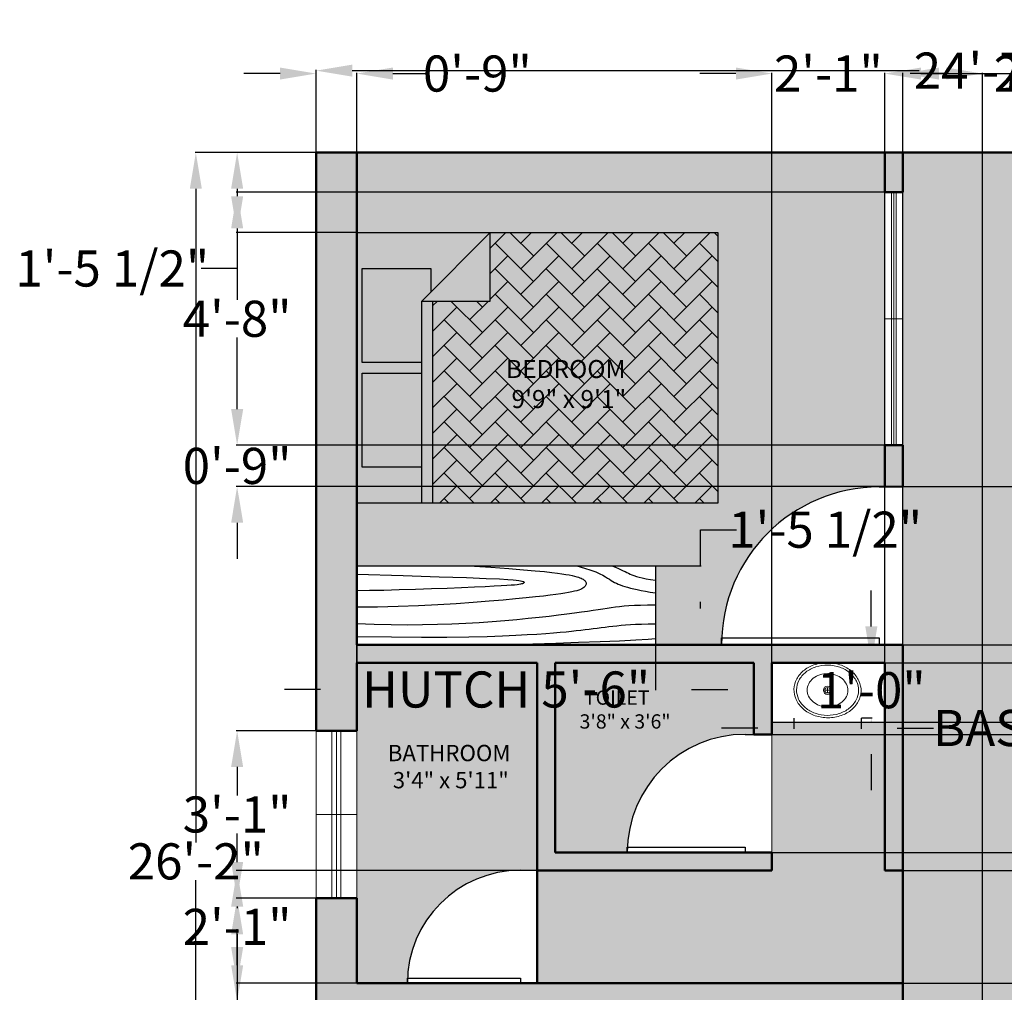
# Model space of a CAD drawing. Units: inches. Extents: x 339 to 824, y 73 to 445.
# Tile 2 of 5: x 387 to 605, y 230 to 445. Entities that reach past the tile are written whole.
import ezdxf

# ---------------------------------------------------------------- set-up
doc = ezdxf.new("R2010")
doc.units = ezdxf.units.IN
doc.header["$MEASUREMENT"] = 0
for name, color, linetype, lineweight in [('A-ANNO-DIMS', 2, 'Continuous', 18), ('A-AREA-IDEN', 7, 'Continuous', 25), ('A-DOOR', 3, 'Continuous', 25), ('A-FLOR-BNDY', 8, 'Continuous', 13), ('A-FLOR-CASE', 7, 'Continuous', 25), ('A-FLOR-FIXT', 9, 'Continuous', 20), ('A-FLOR-PATT', 8, 'Continuous', 13), ('A-FLOR-STRS', 7, 'Continuous', 25), ('A-FLOR-STRS-PATT', 252, 'Continuous', 13), ('A-FURN', 9, 'Continuous', 25), ('A-FURN-FABR-PATT', 7, 'Continuous', 13), ('A-GLAZ', 4, 'Continuous', 18), ('A-WALL', 7, 'Continuous', 50), ('A-WALL-PATT', 1, 'Continuous', 13)]:
    doc.layers.add(name, color=color, linetype=linetype, lineweight=lineweight)
doc.layers.add('A-FURN-PATT', color=251, linetype='Continuous', lineweight=13, true_color=0x6d5f6c)
doc.styles.get("Standard").update_dxf_attribs({"font": 'arial.ttf'})
doc.dimstyles.get("Standard").update_dxf_attribs({"dimtxt": 8, "dimasz": 8, "dimexe": 0.18, "dimexo": 0.0625, "dimgap": 0.09, "dimtad": 0, "dimtih": 1, "dimtoh": 1, "dimdec": 0, "dimzin": 0, "dimdsep": 46, "dimlunit": 3, "dimtxsty": 'Standard', "dimcen": 0.09, "dimadec": 0, "dimazin": 0, "dimtfac": 1, "dimtdec": 0, "dimtofl": 0, "dimtmove": 0, "dimatfit": 3, "dimfxl": 1, "dimtolj": 1, "dimtzin": 0, "dimarcsym": 0})

# ---------------------------------------------------------------- blocks, each defined once
blk = doc.blocks.new('*U2')
for p, q in [((0, 0), (0, -6)), ((40, 0), (40, -6))]:
    blk.add_line(p, q)
blk.add_lwpolyline([(0, 0), (0, 40), (1.75, 40), (1.75, 0)], close=True)
blk.add_arc((0, 0), 40, 0, 90)
blk = doc.blocks.new('Sink - Oval top')
for p, q in [((-1, 0), (1, 0)), ((0, 1), (0, -1))]:
    blk.add_line(p, q)
for points in [[(-12.23, 0.39, 0.117634), (-11.46, -3.36, 0.104469), (-8.88, -6.8, 0.090016), (-5.08, -9.07, 0.08192), (-0.32, -10.02, 0.08192), (4.49, -9.38, 0.090016), (8.42, -7.36, 0.104469), (11.22, -4.09, 0.117634), (12.23, -0.39, 0.117634), (11.46, 3.36, 0.104469), (8.88, 6.8, 0.090016), (5.08, 9.07, 0.08192), (0.32, 10.02, 0.08192), (-4.49, 9.38, 0.090016), (-8.42, 7.36, 0.104469), (-11.22, 4.09, 0.117634)], [(-11.29, 0.16, 0.118622), (-10.52, -3.25, 0.104678), (-8.07, -6.36, 0.089562), (-4.54, -8.37, 0.081185), (-0.13, -9.15, 0.081185), (4.3, -8.49, 0.089562), (7.89, -6.58, 0.104678), (10.42, -3.55, 0.118622), (11.29, -0.16, 0.118622), (10.52, 3.25, 0.104678), (8.07, 6.36, 0.089562), (4.54, 8.37, 0.081185), (0.13, 9.15, 0.081185), (-4.3, 8.49, 0.089562), (-7.89, 6.58, 0.104678), (-10.42, 3.55, 0.118622)], [(-7.42, 0.08, 0.118283), (-6.91, -2.17, 0.104607), (-5.29, -4.21, 0.089718), (-2.97, -5.53, 0.081436), (-0.07, -6.04, 0.081436), (2.84, -5.59, 0.089718), (5.2, -4.33, 0.104607), (6.86, -2.32, 0.118283), (7.42, -0.08, 0.118283), (6.91, 2.17, 0.104607), (5.29, 4.21, 0.089718), (2.97, 5.53, 0.081436), (0.07, 6.04, 0.081436), (-2.84, 5.59, 0.089718), (-5.2, 4.33, 0.104607), (-6.86, 2.32, 0.118283)]]:
    blk.add_lwpolyline(points, format="xyb", close=True)
for radius in [1.5, 1]:
    blk.add_circle((0, 0), radius)
blk = doc.blocks.new('Bed - Queen')
for p, q in [((0, -80.00003), (0, 0)), ((0, 0), (59.99999, 0)), ((59.99999, 0), (59.99999, -80.00003)), ((7.99999, -1.2), (28.79998, -1.2)), ((7.99999, -14.4), (7.99999, -1.2)), ((28.79998, -1.2), (28.79998, -14.4)), ((31.19999, -1.2), (51.99999, -1.2)), ((31.19999, -14.4), (31.19999, -1.2)), ((51.99999, -1.2), (51.99999, -16.4)), ((0, -14.4), (44.8, -14.4)), ((59.99999, -29.6), (44.8, -14.4)), ((44.8, -14.4), (44.8, -29.6)), ((44.8, -16.8), (0, -16.8)), ((51.99999, -16.4), (46.79936, -16.4)), ((44.8, -29.6), (59.99999, -29.6)), ((59.99999, -80.00003), (0, -80.00003))]:
    blk.add_line(p, q)
blk = doc.blocks.new('Hutch - 19 x 72 in.')
for p, q in [((0, -19), (0, 0)), ((0, 0), (71.999994, 0)), ((71.999994, 0), (71.999994, -19)), ((71.999994, -19), (0, -19))]:
    blk.add_line(p, q)
for points in [[(26.99999, 0), (32.30411, -0.35238), (36.66731, -0.66276), (40.20336, -0.93603), (43.02603, -1.17708), (45.2491, -1.39079), (46.98632, -1.58203), (48.35147, -1.7557), (49.45833, -1.91667), (50.40388, -2.06917), (51.21809, -2.21484), (51.91414, -2.35465), (52.5052, -2.48958), (53.00447, -2.6206), (53.42512, -2.7487), (53.78035, -2.87484), (54.08333, -3), (54.34537, -3.12516), (54.57031, -3.2513), (54.76008, -3.37939), (54.91666, -3.51042), (55.04198, -3.64534), (55.13801, -3.78516), (55.2067, -3.93083), (55.24999, -4.08333), (55.26904, -4.24316), (55.26171, -4.40885), (55.22509, -4.57845), (55.15624, -4.75), (55.05224, -4.92155), (54.91015, -5.09115), (54.72704, -5.25684), (54.49999, -5.41667), (54.22493, -5.56934), (53.89322, -5.71615), (53.49511, -5.85905), (53.02083, -6), (52.4606, -6.14095), (51.80468, -6.28385), (51.04329, -6.43066), (50.16666, -6.58333), (49.16007, -6.74381), (47.98892, -6.91406), (46.61368, -7.09603), (44.99478, -7.29167), (43.09268, -7.50293), (40.86783, -7.73177), (38.28067, -7.98014), (35.29166, -8.25), (31.87654, -8.54053), (28.07226, -8.83984), (23.93107, -9.1333), (19.5052, -9.40625), (14.84692, -9.64404), (10.00846, -9.83203), (5.04207, -9.95557), (0, -10)], [(52.99999, 0), (54.87133, -0.53955), (56.39257, -1.03516), (57.61205, -1.48975), (58.57812, -1.90625), (59.3391, -2.2876), (59.94335, -2.63672), (60.4392, -2.95654), (60.87499, -3.25), (61.29247, -3.52002), (61.70702, -3.76953), (62.12743, -4.00146), (62.56249, -4.21875), (63.02099, -4.42432), (63.51171, -4.62109), (64.04345, -4.81201), (64.62499, -5), (65.26489, -5.1875), (65.9707, -5.375), (66.74975, -5.5625), (67.60937, -5.75), (68.55688, -5.9375), (69.5996, -6.125), (70.744867, -6.3125), (71.999994, -6.5)], [(61.49999, 0), (62.35961, -0.35254), (63.08007, -0.66406), (63.68627, -0.94043), (64.20312, -1.1875), (64.65551, -1.41113), (65.06835, -1.61719), (65.46655, -1.81152), (65.87499, -2), (66.31762, -2.1875), (66.81445, -2.375), (67.38452, -2.5625), (68.04687, -2.75), (68.82055, -2.9375), (69.7246, -3.125), (70.77807, -3.3125), (71.999994, -3.5)], [(0, -2), (11.2006, -2.34123), (19.90169, -2.62044), (26.43969, -2.84595), (31.15103, -3.02604), (34.37214, -3.16903), (36.43945, -3.2832), (37.68936, -3.37687), (38.45833, -3.45833), (39.02937, -3.53459), (39.472, -3.60742), (39.80232, -3.67733), (40.03645, -3.74479), (40.1905, -3.8103), (40.28059, -3.87435), (40.32283, -3.93742), (40.33333, -4), (40.32405, -4.0625), (40.29036, -4.125), (40.22346, -4.1875), (40.11458, -4.25), (39.95491, -4.3125), (39.73567, -4.375), (39.44807, -4.4375), (39.08333, -4.5), (38.62491, -4.56282), (38.02538, -4.6276), (37.22957, -4.69629), (36.18228, -4.77083), (34.82836, -4.85319), (33.11262, -4.94531), (30.97989, -5.04915), (28.37499, -5.16667), (25.27416, -5.29818), (21.77929, -5.4375), (18.02368, -5.57682), (14.14062, -5.70833), (10.26342, -5.82422), (6.52539, -5.91667), (3.05981, -5.97786), (0, -6)], [(71.999994, -9.5), (70.071934, -9.51147), (68.38801, -9.54492), (66.91113, -9.59888), (65.60416, -9.67187), (64.43001, -9.76245), (63.35156, -9.86914), (62.3317, -9.99048), (61.33333, -10.125), (60.32128, -10.27157), (59.26822, -10.43034), (58.14876, -10.60181), (56.93749, -10.78646), (55.60904, -10.98478), (54.13801, -11.19726), (52.49902, -11.4244), (50.66666, -11.66667), (48.62239, -11.92358), (46.37499, -12.19075), (43.9401, -12.46281), (41.33333, -12.73437), (38.57031, -13.00008), (35.66666, -13.25456), (32.63801, -13.49243), (29.49999, -13.70833), (26.26367, -13.89689), (22.92187, -14.05273), (19.46289, -14.17049), (15.875, -14.24479), (12.14648, -14.27026), (8.26562, -14.24154), (4.2207, -14.15324), (0, -14)], [(0, -17), (8.37556, -17.14274), (15.58268, -17.20443), (21.74194, -17.19775), (26.97395, -17.13542), (31.39933, -17.03011), (35.13866, -16.89453), (38.31257, -16.74137), (41.04166, -16.58333), (43.4322, -16.43083), (45.5332, -16.28516), (47.37931, -16.14534), (49.0052, -16.01042), (50.44555, -15.87939), (51.73502, -15.7513), (52.90828, -15.62516), (53.99999, -15.5), (55.04044, -15.37508), (56.04231, -15.25065), (57.01391, -15.1272), (57.96353, -15.00521), (58.89949, -14.88517), (59.83007, -14.76758), (60.76358, -14.65291), (61.70833, -14.54167), (62.6752, -14.43465), (63.68554, -14.33398), (64.76326, -14.24211), (65.93229, -14.16146), (67.21655, -14.09448), (68.63997, -14.04362), (70.226475, -14.01131), (71.999994, -14)], [(36.99999, -19), (42.40038, -18.8125), (47.95312, -18.625), (53.43554, -18.4375), (58.62499, -18.25), (63.29882, -18.0625), (67.23437, -17.875), (70.208978, -17.6875), (71.999994, -17.5)]]:
    blk.add_lwpolyline(points)
blk = doc.blocks.new('*D11')
at = {"layer": 'A-ANNO-DIMS', "color": 0, "lineweight": -2, "transparency": 16777216}
for p, q in [((452.48, 416.12), (452.48, 434.39)), ((460.48, 434.21), (586.08, 434.21)), ((739.48, 434.21), (613.88, 434.21)), ((747.48, 416.12), (747.48, 434.39))]:
    blk.add_line(p, q, dxfattribs=at)
at = {"layer": 'A-ANNO-DIMS', "color": 0, "transparency": 16777216}
for points in [[(460.48, 435.54), (460.48, 432.88), (452.48, 434.21)], [(739.48, 435.54), (739.48, 432.88), (747.48, 434.21)]]:
    blk.add_solid(points, dxfattribs=at)
at = {"layer": 'Defpoints', "color": 0, "transparency": 16777216}
for p in [(747.48, 434.21), (452.48, 416.06), (747.48, 416.06)]:
    blk.add_point(p, dxfattribs=at)
at = {"layer": 'A-ANNO-DIMS', "color": 0, "transparency": 16777216, "insert": (599.98, 434.21), "char_height": 8, "attachment_point": 5}
blk.add_mtext('\\A1;24\'-7"', dxfattribs=at)
blk = doc.blocks.new('*D12')
at = {"layer": 'A-ANNO-DIMS', "color": 0, "lineweight": -2, "transparency": 16777216}
for p, q in [((452.42, 416.06), (425.65, 416.06)), ((425.83, 408.06), (425.83, 263.23)), ((425.83, 110.06), (425.83, 254.89)), ((452.42, 102.06), (425.65, 102.06))]:
    blk.add_line(p, q, dxfattribs=at)
at = {"layer": 'A-ANNO-DIMS', "color": 0, "transparency": 16777216}
for points in [[(424.5, 408.06), (427.16, 408.06), (425.83, 416.06)], [(424.5, 110.06), (427.16, 110.06), (425.83, 102.06)]]:
    blk.add_solid(points, dxfattribs=at)
at = {"layer": 'Defpoints', "color": 0, "transparency": 16777216}
for p in [(452.48, 416.06), (425.83, 102.06), (452.48, 102.06)]:
    blk.add_point(p, dxfattribs=at)
at = {"layer": 'A-ANNO-DIMS', "color": 0, "transparency": 16777216, "insert": (425.83, 259.06), "char_height": 8, "attachment_point": 5}
blk.add_mtext('\\A1;26\'-2"', dxfattribs=at)
blk = doc.blocks.new('*D18')
at = {"layer": 'A-ANNO-DIMS', "color": 0, "lineweight": -2, "transparency": 16777216}
for p, q in [((461.48, 307), (461.48, 296.95)), ((527.68, 307), (527.68, 296.95)), ((453.48, 297.13), (445.48, 297.13)), ((535.68, 297.13), (543.68, 297.13))]:
    blk.add_line(p, q, dxfattribs=at)
at = {"layer": 'A-ANNO-DIMS', "color": 0, "transparency": 16777216}
for points in [[(453.48, 298.46), (453.48, 295.8), (461.48, 297.13)], [(535.68, 298.46), (535.68, 295.8), (527.68, 297.13)]]:
    blk.add_solid(points, dxfattribs=at)
at = {"layer": 'Defpoints', "color": 0, "transparency": 16777216}
for p in [(461.48, 307.06), (527.68, 307.06), (527.68, 297.13)]:
    blk.add_point(p, dxfattribs=at)
at = {"layer": 'A-ANNO-DIMS', "color": 0, "transparency": 16777216, "insert": (494.58, 297.13), "char_height": 8, "attachment_point": 5}
blk.add_mtext('\\A1;HUTCH 5\'-6"', dxfattribs=at)
blk = doc.blocks.new('*D19')
at = {"layer": 'A-ANNO-DIMS', "color": 0, "lineweight": -2, "transparency": 16777216}
for p, q in [((537.61, 324.53), (537.61, 332.53)), ((537.61, 332.53), (545.61, 332.53)), ((527.75, 324.53), (537.79, 324.53)), ((537.61, 315.06), (537.61, 316.53)), ((527.75, 307.06), (537.79, 307.06))]:
    blk.add_line(p, q, dxfattribs=at)
at = {"layer": 'A-ANNO-DIMS', "color": 0, "transparency": 16777216}
for points in [[(536.28, 316.53), (538.95, 316.53), (537.61, 324.53)], [(536.28, 315.06), (538.95, 315.06), (537.61, 307.06)]]:
    blk.add_solid(points, dxfattribs=at)
at = {"layer": 'Defpoints', "color": 0, "transparency": 16777216}
for p in [(527.68, 324.53), (537.61, 324.53), (527.68, 307.06)]:
    blk.add_point(p, dxfattribs=at)
at = {"layer": 'A-ANNO-DIMS', "color": 0, "transparency": 16777216, "insert": (565.28, 332.53), "char_height": 8, "attachment_point": 5}
blk.add_mtext('\\A1;1\'-5 1/2"', dxfattribs=at)
blk = doc.blocks.new('*D20')
at = {"layer": 'A-ANNO-DIMS', "color": 0, "lineweight": -2, "transparency": 16777216}
for p, q in [((558.32, 290.78), (558.32, 288.42)), ((573.25, 290.78), (573.25, 288.42)), ((550.32, 288.6), (542.32, 288.6)), ((581.25, 288.6), (589.25, 288.6))]:
    blk.add_line(p, q, dxfattribs=at)
at = {"layer": 'A-ANNO-DIMS', "color": 0, "transparency": 16777216}
for points in [[(550.32, 289.94), (550.32, 287.27), (558.32, 288.6)], [(581.25, 289.94), (581.25, 287.27), (573.25, 288.6)]]:
    blk.add_solid(points, dxfattribs=at)
at = {"layer": 'Defpoints', "color": 0, "transparency": 16777216}
for p in [(558.32, 290.84), (573.25, 290.84), (573.25, 288.6)]:
    blk.add_point(p, dxfattribs=at)
at = {"layer": 'A-ANNO-DIMS', "color": 0, "transparency": 16777216, "insert": (618.12, 288.6), "char_height": 8, "attachment_point": 5}
blk.add_mtext('\\A1;BASIN 1\'-3"', dxfattribs=at)
blk = doc.blocks.new('*D21')
at = {"layer": 'A-ANNO-DIMS', "color": 0, "lineweight": -2, "transparency": 16777216}
for p, q in [((575.49, 311.09), (575.49, 319.09)), ((573.32, 303.09), (575.67, 303.09)), ((573.32, 290.84), (575.67, 290.84)), ((575.49, 282.84), (575.49, 274.84))]:
    blk.add_line(p, q, dxfattribs=at)
at = {"layer": 'A-ANNO-DIMS', "color": 0, "transparency": 16777216}
for points in [[(574.16, 311.09), (576.83, 311.09), (575.49, 303.09)], [(574.16, 282.84), (576.83, 282.84), (575.49, 290.84)]]:
    blk.add_solid(points, dxfattribs=at)
at = {"layer": 'Defpoints', "color": 0, "transparency": 16777216}
for p in [(573.25, 303.09), (575.49, 303.09), (573.25, 290.84)]:
    blk.add_point(p, dxfattribs=at)
at = {"layer": 'A-ANNO-DIMS', "color": 0, "transparency": 16777216, "insert": (575.49, 296.97), "char_height": 8, "attachment_point": 5}
blk.add_mtext('\\A1;1\'-0"', dxfattribs=at)
blk = doc.blocks.new('*D34')
at = {"layer": 'A-ANNO-DIMS', "color": 0, "lineweight": -2, "transparency": 16777216}
for p, q in [((452.42, 250.91), (434.8, 250.91)), ((434.98, 242.91), (434.98, 180.66)), ((434.98, 110.06), (434.98, 172.31)), ((452.42, 102.06), (434.8, 102.06))]:
    blk.add_line(p, q, dxfattribs=at)
at = {"layer": 'A-ANNO-DIMS', "color": 0, "transparency": 16777216}
for points in [[(433.65, 242.91), (436.32, 242.91), (434.98, 250.91)], [(433.65, 110.06), (436.32, 110.06), (434.98, 102.06)]]:
    blk.add_solid(points, dxfattribs=at)
at = {"layer": 'Defpoints', "color": 0, "transparency": 16777216}
for p in [(434.98, 250.91), (452.48, 250.91), (452.48, 102.06)]:
    blk.add_point(p, dxfattribs=at)
at = {"layer": 'A-ANNO-DIMS', "color": 0, "transparency": 16777216, "insert": (434.98, 176.48), "char_height": 8, "attachment_point": 5}
blk.add_mtext('\\A1;12\'-5"', dxfattribs=at)
blk = doc.blocks.new('*D35')
at = {"layer": 'A-ANNO-DIMS', "color": 0, "lineweight": -2, "transparency": 16777216}
for p, q in [((452.42, 287.98), (434.8, 287.98)), ((434.98, 279.98), (434.98, 273.62)), ((434.98, 258.91), (434.98, 265.27)), ((452.42, 250.91), (434.8, 250.91))]:
    blk.add_line(p, q, dxfattribs=at)
at = {"layer": 'A-ANNO-DIMS', "color": 0, "transparency": 16777216}
for points in [[(433.65, 279.98), (436.32, 279.98), (434.98, 287.98)], [(433.65, 258.91), (436.32, 258.91), (434.98, 250.91)]]:
    blk.add_solid(points, dxfattribs=at)
at = {"layer": 'Defpoints', "color": 0, "transparency": 16777216}
for p in [(434.98, 287.98), (452.48, 287.98), (452.48, 250.91)]:
    blk.add_point(p, dxfattribs=at)
at = {"layer": 'A-ANNO-DIMS', "color": 0, "transparency": 16777216, "insert": (434.98, 269.45), "char_height": 8, "attachment_point": 5}
blk.add_mtext('\\A1;3\'-1"', dxfattribs=at)
blk = doc.blocks.new('*D38')
at = {"layer": 'A-ANNO-DIMS', "color": 0, "lineweight": -2, "transparency": 16777216}
for p, q in [((592.11, 433.56), (584.11, 433.56)), ((600.11, 213.12), (600.11, 433.74)), ((635.29, 213.12), (635.29, 433.74)), ((643.29, 433.56), (651.29, 433.56))]:
    blk.add_line(p, q, dxfattribs=at)
at = {"layer": 'A-ANNO-DIMS', "color": 0, "transparency": 16777216}
for points in [[(592.11, 434.89), (592.11, 432.23), (600.11, 433.56)], [(643.29, 434.89), (643.29, 432.23), (635.29, 433.56)]]:
    blk.add_solid(points, dxfattribs=at)
at = {"layer": 'Defpoints', "color": 0, "transparency": 16777216}
for p in [(635.29, 433.56), (600.11, 213.06), (635.29, 213.06)]:
    blk.add_point(p, dxfattribs=at)
at = {"layer": 'A-ANNO-DIMS', "color": 0, "transparency": 16777216, "insert": (617.7, 433.56), "char_height": 8, "attachment_point": 5}
blk.add_mtext('\\A1;2\'-11"', dxfattribs=at)
blk = doc.blocks.new('*D41')
at = {"layer": 'A-ANNO-DIMS', "color": 0, "lineweight": -2, "transparency": 16777216}
for p, q in [((582.55, 342.06), (765.16, 342.06)), ((764.98, 334.06), (764.98, 328.67)), ((764.98, 315.06), (764.98, 320.45)), ((582.55, 307.06), (765.16, 307.06))]:
    blk.add_line(p, q, dxfattribs=at)
at = {"layer": 'A-ANNO-DIMS', "color": 0, "transparency": 16777216}
for points in [[(763.65, 334.06), (766.32, 334.06), (764.98, 342.06)], [(763.65, 315.06), (766.32, 315.06), (764.98, 307.06)]]:
    blk.add_solid(points, dxfattribs=at)
at = {"layer": 'Defpoints', "color": 0, "transparency": 16777216}
for p in [(582.48, 342.06), (582.48, 307.06), (764.98, 307.06)]:
    blk.add_point(p, dxfattribs=at)
at = {"layer": 'A-ANNO-DIMS', "color": 0, "transparency": 16777216, "insert": (764.98, 324.56), "char_height": 8, "attachment_point": 5}
blk.add_mtext('\\A1;2\'-11"', dxfattribs=at)
blk = doc.blocks.new('*D42')
at = {"layer": 'A-ANNO-DIMS', "color": 0, "lineweight": -2, "transparency": 16777216}
for p, q in [((582.55, 257.06), (765.16, 257.06)), ((764.98, 249.06), (764.98, 248.67)), ((764.98, 240.06), (764.98, 240.45)), ((582.55, 232.06), (765.16, 232.06))]:
    blk.add_line(p, q, dxfattribs=at)
at = {"layer": 'A-ANNO-DIMS', "color": 0, "transparency": 16777216}
for points in [[(763.65, 249.06), (766.32, 249.06), (764.98, 257.06)], [(763.65, 240.06), (766.32, 240.06), (764.98, 232.06)]]:
    blk.add_solid(points, dxfattribs=at)
at = {"layer": 'Defpoints', "color": 0, "transparency": 16777216}
for p in [(582.48, 257.06), (582.48, 232.06), (764.98, 232.06)]:
    blk.add_point(p, dxfattribs=at)
at = {"layer": 'A-ANNO-DIMS', "color": 0, "transparency": 16777216, "insert": (764.98, 244.56), "char_height": 8, "attachment_point": 5}
blk.add_mtext('\\A1;2\'-1"', dxfattribs=at)
blk = doc.blocks.new('*D43')
at = {"layer": 'A-ANNO-DIMS', "color": 0, "lineweight": -2, "transparency": 16777216}
for p, q in [((501.42, 257.06), (434.8, 257.06)), ((434.98, 249.06), (434.98, 248.67)), ((434.98, 240.06), (434.98, 240.45)), ((501.42, 232.06), (434.8, 232.06))]:
    blk.add_line(p, q, dxfattribs=at)
at = {"layer": 'A-ANNO-DIMS', "color": 0, "transparency": 16777216}
for points in [[(433.65, 249.06), (436.32, 249.06), (434.98, 257.06)], [(433.65, 240.06), (436.32, 240.06), (434.98, 232.06)]]:
    blk.add_solid(points, dxfattribs=at)
at = {"layer": 'Defpoints', "color": 0, "transparency": 16777216}
for p in [(434.98, 257.06), (501.48, 257.06), (501.48, 232.06)]:
    blk.add_point(p, dxfattribs=at)
at = {"layer": 'A-ANNO-DIMS', "color": 0, "transparency": 16777216, "insert": (434.98, 244.56), "char_height": 8, "attachment_point": 5}
blk.add_mtext('\\A1;2\'-1"', dxfattribs=at)
blk = doc.blocks.new('*D44')
at = {"layer": 'A-ANNO-DIMS', "color": 0, "lineweight": -2, "transparency": 16777216}
for p, q in [((553.55, 287.19), (765.16, 287.19)), ((764.98, 279.19), (764.98, 278.23)), ((764.98, 269.06), (764.98, 270.02)), ((553.55, 261.06), (765.16, 261.06))]:
    blk.add_line(p, q, dxfattribs=at)
at = {"layer": 'A-ANNO-DIMS', "color": 0, "transparency": 16777216}
for points in [[(763.65, 279.19), (766.32, 279.19), (764.98, 287.19)], [(763.65, 269.06), (766.32, 269.06), (764.98, 261.06)]]:
    blk.add_solid(points, dxfattribs=at)
at = {"layer": 'Defpoints', "color": 0, "transparency": 16777216}
for p in [(553.48, 287.19), (764.98, 287.19), (553.48, 261.06)]:
    blk.add_point(p, dxfattribs=at)
at = {"layer": 'A-ANNO-DIMS', "color": 0, "transparency": 16777216, "insert": (764.98, 274.12), "char_height": 8, "attachment_point": 5}
blk.add_mtext('\\A1;2\'-2"', dxfattribs=at)
blk = doc.blocks.new('*D45')
at = {"layer": 'A-ANNO-DIMS', "color": 0, "lineweight": -2, "transparency": 16777216}
for p, q in [((545.48, 433.56), (537.48, 433.56)), ((553.48, 303.12), (553.48, 433.74)), ((578.48, 303.12), (578.48, 433.74)), ((586.48, 433.56), (594.48, 433.56))]:
    blk.add_line(p, q, dxfattribs=at)
at = {"layer": 'A-ANNO-DIMS', "color": 0, "transparency": 16777216}
for points in [[(545.48, 434.89), (545.48, 432.23), (553.48, 433.56)], [(586.48, 434.89), (586.48, 432.23), (578.48, 433.56)]]:
    blk.add_solid(points, dxfattribs=at)
at = {"layer": 'Defpoints', "color": 0, "transparency": 16777216}
for p in [(578.48, 433.56), (553.48, 303.06), (578.48, 303.06)]:
    blk.add_point(p, dxfattribs=at)
at = {"layer": 'A-ANNO-DIMS', "color": 0, "transparency": 16777216, "insert": (565.98, 433.56), "char_height": 8, "attachment_point": 5}
blk.add_mtext('\\A1;2\'-1"', dxfattribs=at)
blk = doc.blocks.new('*D46')
at = {"layer": 'A-ANNO-DIMS', "color": 0, "lineweight": -2, "transparency": 16777216}
for p, q in [((764.98, 311.06), (764.98, 319.06)), ((578.55, 303.06), (765.16, 303.06)), ((578.55, 289.86), (765.16, 289.86)), ((764.98, 281.86), (764.98, 273.86))]:
    blk.add_line(p, q, dxfattribs=at)
at = {"layer": 'A-ANNO-DIMS', "color": 0, "transparency": 16777216}
for points in [[(763.65, 311.06), (766.32, 311.06), (764.98, 303.06)], [(763.65, 281.86), (766.32, 281.86), (764.98, 289.86)]]:
    blk.add_solid(points, dxfattribs=at)
at = {"layer": 'Defpoints', "color": 0, "transparency": 16777216}
for p in [(578.48, 303.06), (578.48, 289.86), (764.98, 289.86)]:
    blk.add_point(p, dxfattribs=at)
at = {"layer": 'A-ANNO-DIMS', "color": 0, "transparency": 16777216, "insert": (764.98, 296.46), "char_height": 8, "attachment_point": 5}
blk.add_mtext('\\A1;1\'-1"', dxfattribs=at)
blk = doc.blocks.new('*D47')
at = {"layer": 'A-ANNO-DIMS', "color": 0, "lineweight": -2, "transparency": 16777216}
for p, q in [((582.42, 407.26), (434.8, 407.26)), ((434.98, 399.26), (434.98, 383.42)), ((434.98, 359.23), (434.98, 375.07)), ((582.42, 351.23), (434.8, 351.23))]:
    blk.add_line(p, q, dxfattribs=at)
at = {"layer": 'A-ANNO-DIMS', "color": 0, "transparency": 16777216}
for points in [[(433.65, 399.26), (436.32, 399.26), (434.98, 407.26)], [(433.65, 359.23), (436.32, 359.23), (434.98, 351.23)]]:
    blk.add_solid(points, dxfattribs=at)
at = {"layer": 'Defpoints', "color": 0, "transparency": 16777216}
for p in [(582.48, 407.26), (434.98, 351.23), (582.48, 351.23)]:
    blk.add_point(p, dxfattribs=at)
at = {"layer": 'A-ANNO-DIMS', "color": 0, "transparency": 16777216, "insert": (434.98, 379.25), "char_height": 8, "attachment_point": 5}
blk.add_mtext('\\A1;4\'-8"', dxfattribs=at)
blk = doc.blocks.new('*D48')
at = {"layer": 'A-ANNO-DIMS', "color": 0, "lineweight": -2, "transparency": 16777216}
for p, q in [((434.98, 359.23), (434.98, 367.23)), ((582.42, 351.23), (434.8, 351.23)), ((582.42, 342.06), (434.8, 342.06)), ((434.98, 334.06), (434.98, 326.06))]:
    blk.add_line(p, q, dxfattribs=at)
at = {"layer": 'A-ANNO-DIMS', "color": 0, "transparency": 16777216}
for points in [[(433.65, 359.23), (436.32, 359.23), (434.98, 351.23)], [(433.65, 334.06), (436.32, 334.06), (434.98, 342.06)]]:
    blk.add_solid(points, dxfattribs=at)
at = {"layer": 'Defpoints', "color": 0, "transparency": 16777216}
for p in [(582.48, 351.23), (434.98, 342.06), (582.48, 342.06)]:
    blk.add_point(p, dxfattribs=at)
at = {"layer": 'A-ANNO-DIMS', "color": 0, "transparency": 16777216, "insert": (434.98, 346.65), "char_height": 8, "attachment_point": 5}
blk.add_mtext('\\A1;0\'-9"', dxfattribs=at)
blk = doc.blocks.new('*D54')
at = {"layer": 'A-ANNO-DIMS', "color": 0, "lineweight": -2, "transparency": 16777216}
for p, q in [((582.48, 416.12), (582.48, 433.74)), ((590.48, 433.56), (610, 433.56)), ((618, 416.12), (618, 433.74)), ((618, 433.56), (626, 433.56))]:
    blk.add_line(p, q, dxfattribs=at)
at = {"layer": 'A-ANNO-DIMS', "color": 0, "transparency": 16777216}
for points in [[(590.48, 434.89), (590.48, 432.23), (582.48, 433.56)], [(610, 434.89), (610, 432.23), (618, 433.56)]]:
    blk.add_solid(points, dxfattribs=at)
at = {"layer": 'Defpoints', "color": 0, "transparency": 16777216}
for p in [(618, 433.56), (582.48, 416.06), (618, 416.06)]:
    blk.add_point(p, dxfattribs=at)
at = {"layer": 'A-ANNO-DIMS', "color": 0, "transparency": 16777216, "insert": (649.22, 433.56), "char_height": 8, "attachment_point": 5}
blk.add_mtext('\\A1;2\'-11 1/2"', dxfattribs=at)
blk = doc.blocks.new('*D55')
at = {"layer": 'A-ANNO-DIMS', "color": 0, "lineweight": -2, "transparency": 16777216}
for p, q in [((582.48, 213.12), (582.48, 433.74)), ((590.48, 433.56), (592.11, 433.56)), ((600.11, 213.12), (600.11, 433.74)), ((600.11, 433.56), (608.11, 433.56))]:
    blk.add_line(p, q, dxfattribs=at)
at = {"layer": 'A-ANNO-DIMS', "color": 0, "transparency": 16777216}
for points in [[(590.48, 434.89), (590.48, 432.23), (582.48, 433.56)], [(592.11, 434.89), (592.11, 432.23), (600.11, 433.56)]]:
    blk.add_solid(points, dxfattribs=at)
at = {"layer": 'Defpoints', "color": 0, "transparency": 16777216}
for p in [(600.11, 433.56), (582.48, 213.06), (600.11, 213.06)]:
    blk.add_point(p, dxfattribs=at)
at = {"layer": 'A-ANNO-DIMS', "color": 0, "transparency": 16777216, "insert": (627.78, 433.56), "char_height": 8, "attachment_point": 5}
blk.add_mtext('\\A1;1\'-5 1/2"', dxfattribs=at)
blk = doc.blocks.new('*D59')
at = {"layer": 'A-ANNO-DIMS', "color": 0, "lineweight": -2, "transparency": 16777216}
for p, q in [((444.48, 433.56), (436.48, 433.56)), ((452.48, 288.05), (452.48, 433.74)), ((461.48, 288.05), (461.48, 433.74)), ((469.48, 433.56), (477.48, 433.56))]:
    blk.add_line(p, q, dxfattribs=at)
at = {"layer": 'A-ANNO-DIMS', "color": 0, "transparency": 16777216}
for points in [[(444.48, 434.89), (444.48, 432.23), (452.48, 433.56)], [(469.48, 434.89), (469.48, 432.23), (461.48, 433.56)]]:
    blk.add_solid(points, dxfattribs=at)
at = {"layer": 'Defpoints', "color": 0, "transparency": 16777216}
for p in [(461.48, 433.56), (452.48, 287.98), (461.48, 287.98)]:
    blk.add_point(p, dxfattribs=at)
at = {"layer": 'A-ANNO-DIMS', "color": 0, "transparency": 16777216, "insert": (488.21, 433.56), "char_height": 8, "attachment_point": 5}
blk.add_mtext('\\A1;0\'-9"', dxfattribs=at)
blk = doc.blocks.new('*D61')
at = {"layer": 'A-ANNO-DIMS', "color": 0, "lineweight": -2, "transparency": 16777216}
for p, q in [((461.42, 416.06), (434.8, 416.06)), ((434.98, 408.06), (434.98, 406.38)), ((461.42, 398.38), (434.8, 398.38)), ((434.98, 398.38), (434.98, 390.38)), ((434.98, 390.38), (426.98, 390.38))]:
    blk.add_line(p, q, dxfattribs=at)
at = {"layer": 'A-ANNO-DIMS', "color": 0, "transparency": 16777216}
for points in [[(433.65, 408.06), (436.32, 408.06), (434.98, 416.06)], [(433.65, 406.38), (436.32, 406.38), (434.98, 398.38)]]:
    blk.add_solid(points, dxfattribs=at)
at = {"layer": 'Defpoints', "color": 0, "transparency": 16777216}
for p in [(461.48, 416.06), (434.98, 398.38), (461.48, 398.38)]:
    blk.add_point(p, dxfattribs=at)
at = {"layer": 'A-ANNO-DIMS', "color": 0, "transparency": 16777216, "insert": (407.32, 390.38), "char_height": 8, "attachment_point": 5}
blk.add_mtext('\\A1;1\'-5 1/2"', dxfattribs=at)
blk = doc.blocks.new('*D62')
at = {"layer": 'A-ANNO-DIMS', "color": 0, "lineweight": -2, "transparency": 16777216}
for p, q in [((434.98, 236.06), (434.98, 244.06)), ((461.42, 228.06), (434.8, 228.06)), ((461.42, 218.85), (434.8, 218.85)), ((434.98, 210.85), (434.98, 202.85))]:
    blk.add_line(p, q, dxfattribs=at)
at = {"layer": 'A-ANNO-DIMS', "color": 0, "transparency": 16777216}
for points in [[(433.65, 236.06), (436.32, 236.06), (434.98, 228.06)], [(433.65, 210.85), (436.32, 210.85), (434.98, 218.85)]]:
    blk.add_solid(points, dxfattribs=at)
at = {"layer": 'Defpoints', "color": 0, "transparency": 16777216}
for p in [(461.48, 228.06), (434.98, 218.85), (461.48, 218.85)]:
    blk.add_point(p, dxfattribs=at)
at = {"layer": 'A-ANNO-DIMS', "color": 0, "transparency": 16777216, "insert": (434.98, 223.45), "char_height": 8, "attachment_point": 5}
blk.add_mtext('\\A1;0\'-9"', dxfattribs=at)

msp = doc.modelspace()

# ---------------------------------------------------------------- hatches: boundary and pattern name
at = {"layer": 'A-FLOR-PATT'}
h = msp.add_hatch(color=256, dxfattribs=at)
h.dxf.hatch_style = 1
h.paths.add_polyline_path([(541.48, 338.38), (461.48, 338.38), (461.48, 324.53), (527.68, 324.53), (527.68, 307.06), (542.32, 307.06), (542.32, 308.59), (542.35, 308.59, -0.401453), (577.24, 341.99), (578.48, 341.99), (578.48, 351.23), (578.48, 407.26), (578.48, 416.06), (461.48, 416.06), (461.48, 398.38), (541.48, 398.38)])
h = msp.add_hatch(color=256, dxfattribs=at)
h.dxf.hatch_style = 1
h.paths.add_polyline_path([(661.42, 241.56), (665.51, 241.56, -0.414214), (667.55, 243.6), (678.83, 243.6, -0.414214), (680.87, 241.56, -0.414214), (682.91, 243.6), (696.76, 243.6, -0.414214), (698.8, 241.56, -0.414214), (700.84, 243.6), (714.97, 243.6, -0.412935), (717.02, 241.56, -0.410727), (719.02, 243.61, -0.419077), (716.95, 245.66), (716.95, 259.06, -0.414214), (718.99, 261.11, -0.414214), (716.95, 263.15), (716.95, 274.6, -0.414214), (718.99, 276.64), (718.99, 280.73, -0.414214), (720.01, 281.75), (743.48, 281.75), (743.48, 293.36), (743.48, 299.72), (741.87, 299.72), (741.87, 299.75, -0.401453), (706.66, 336.54), (706.66, 342.06), (582.48, 342.06), (582.48, 307.06), (582.48, 217.06), (635.29, 217.06), (660.4, 217.06), (660.4, 240.53, -0.414214)])
h.paths.add_polyline_path([(639.94, 279.04), (679.09, 279.04), (679.09, 293.92), (639.94, 293.92)], flags=24)
h = msp.add_hatch(color=256, dxfattribs=at)
h.dxf.hatch_style = 1
h.paths.add_polyline_path([(501.48, 303.06), (461.48, 303.06), (461.48, 287.98), (461.48, 250.91), (461.48, 232.06), (472.7, 232.06), (472.7, 233.16), (472.72, 233.16, -0.401453), (497.73, 257.09), (501.48, 257.09)])
h.paths.add_polyline_path([(467.1, 273.2), (497.99, 273.2), (497.99, 286.65), (467.1, 286.65)], flags=24)
h = msp.add_hatch(color=256, dxfattribs=at)
h.dxf.hatch_style = 1
h.paths.add_polyline_path([(501.48, 303.06), (461.48, 303.06), (461.48, 287.98), (461.48, 250.91), (461.48, 232.06), (472.7, 232.06), (472.7, 233.16), (472.72, 233.16, -0.401453), (497.73, 257.09), (501.48, 257.09)])
h.paths.add_polyline_path([(467.1, 273.2), (497.99, 273.2), (497.99, 286.65), (467.1, 286.65)], flags=24)
h = msp.add_hatch(color=256, dxfattribs=at)
h.dxf.hatch_style = 1
h.paths.add_polyline_path([(547.56, 287.19), (549.48, 287.19), (549.48, 303.06), (505.48, 303.06), (505.48, 261.06), (521.43, 261.06), (521.43, 262.2), (521.46, 262.2, -0.401453)])
h.paths.add_polyline_path([(509.88, 286.68), (530.79, 286.68), (530.79, 298.49), (509.88, 298.49)], flags=24)
h = msp.add_hatch(color=256, dxfattribs=at)
h.dxf.hatch_style = 1
h.paths.add_polyline_path([(505.48, 261.06), (521.43, 261.06), (521.43, 262.2), (521.46, 262.2, -0.401453), (547.56, 287.19), (549.48, 287.19), (549.48, 303.06), (505.48, 303.06)])
h.paths.add_polyline_path([(509.88, 286.68), (530.79, 286.68), (530.79, 298.49), (509.88, 298.49)], flags=24)
h = msp.add_hatch(color=256, dxfattribs=at)
h.dxf.hatch_style = 1
h.paths.add_polyline_path([(501.48, 257.06), (501.48, 232.06), (582.48, 232.06), (582.48, 257.06), (578.48, 257.06), (578.48, 289.86), (553.48, 289.86), (553.48, 287.19), (553.48, 261.06), (553.48, 257.06)])
h = msp.add_hatch(color=256, dxfattribs=at)
h.dxf.hatch_style = 1
h.paths.add_polyline_path([(501.48, 257.06), (501.48, 232.06), (582.48, 232.06), (582.48, 257.06), (578.48, 257.06), (578.48, 289.86), (553.48, 289.86), (553.48, 287.19), (553.48, 261.06), (553.48, 257.06)])
at = {"layer": 'A-FLOR-STRS-PATT'}
h = msp.add_hatch(color=256, dxfattribs=at)
h.dxf.hatch_style = 1
h.paths.add_polyline_path([(582.48, 351.23), (582.48, 342.06), (618, 342.06), (618, 416.06), (582.48, 416.06), (582.48, 407.26)])
at = {"layer": 'A-FURN-FABR-PATT'}
h = msp.add_hatch(dxfattribs=at)
h.set_pattern_fill('AR-HBONE', color=256)
h.paths.add_polyline_path([(541.48, 338.38), (541.48, 398.38), (491.08, 398.38), (491.08, 383.18), (478.28, 383.18), (478.28, 338.38)])
h.paths.add_polyline_path([(493.15, 357.21), (523.93, 357.21), (523.93, 372.1), (493.15, 372.1)], flags=24)
at = {"layer": 'A-FURN-PATT'}
h = msp.add_hatch(color=256, dxfattribs=at)
h.dxf.hatch_style = 1
h.paths.add_polyline_path([(461.48, 398.38), (461.48, 338.38), (475.88, 338.38), (475.88, 346.38), (462.68, 346.38), (462.68, 367.18), (475.88, 367.18), (475.88, 369.58), (462.68, 369.58), (462.68, 390.38), (477.88, 390.38), (477.88, 385.18), (491.08, 398.38)])
h = msp.add_hatch(color=256, dxfattribs=at)
h.dxf.hatch_style = 1
h.paths.add_polyline_path([(475.88, 383.18), (491.08, 383.18), (491.08, 398.38)])
h = msp.add_hatch(color=256, dxfattribs=at)
h.dxf.hatch_style = 1
h.paths.add_polyline_path([(541.48, 338.38), (541.48, 398.38), (491.08, 398.38), (491.08, 383.18), (478.28, 383.18), (478.28, 338.38)])
h.paths.add_polyline_path([(493.15, 357.21), (523.93, 357.21), (523.93, 372.1), (493.15, 372.1)], flags=24)
h = msp.add_hatch(color=256, dxfattribs=at)
h.dxf.hatch_style = 1
h.paths.add_polyline_path([(462.68, 369.58), (475.88, 369.58), (475.88, 383.18), (477.88, 385.18), (477.88, 390.38), (462.68, 390.38)])
h = msp.add_hatch(color=256, dxfattribs=at)
h.dxf.hatch_style = 1
h.paths.add_polyline_path([(478.28, 383.18), (475.88, 383.18), (475.88, 338.38), (478.28, 338.38)])
h = msp.add_hatch(color=256, dxfattribs=at)
h.dxf.hatch_style = 1
h.paths.add_polyline_path([(462.68, 346.38), (475.88, 346.38), (475.88, 367.18), (462.68, 367.18)])
at = {"layer": 'A-WALL-PATT'}
h = msp.add_hatch(color=256, dxfattribs=at)
h.dxf.hatch_style = 1
h.paths.add_polyline_path([(505.48, 261.06), (505.48, 303.06), (549.48, 303.06), (549.48, 287.19), (551.48, 287.19), (553.48, 287.19), (553.48, 303.06), (565.4, 303.06, -0.016107), (565.98, 303.06), (578.48, 303.06), (578.48, 257.06), (582.48, 257.06), (582.48, 307.06), (577.24, 307.06), (542.32, 307.06), (461.48, 307.06), (461.48, 324.53), (461.48, 416.06), (452.48, 416.06), (452.48, 287.98), (461.48, 287.98), (461.48, 303.06), (501.48, 303.06), (501.48, 257.06), (553.48, 257.06), (553.48, 261.06)])
h = msp.add_hatch(color=256, dxfattribs=at)
h.dxf.hatch_style = 1
h.paths.add_polyline_path([(582.48, 416.06), (578.48, 416.06), (578.48, 407.26), (582.48, 407.26)])
h = msp.add_hatch(color=256, dxfattribs=at)
h.dxf.hatch_style = 1
h.paths.add_polyline_path([(582.48, 351.23), (578.48, 351.23), (578.48, 342.06), (582.48, 342.06)])
h = msp.add_hatch(color=256, dxfattribs=at)
h.dxf.hatch_style = 1
h.paths.add_polyline_path([(452.48, 102.06), (495.53, 102.06), (495.53, 106.06), (461.48, 106.06), (461.48, 228.06), (578.48, 228.06), (578.48, 165.46), (578.48, 147.67), (582.48, 147.67), (582.48, 213.06), (600.11, 213.06), (600.11, 215.06), (600.11, 217.06), (582.48, 217.06), (582.48, 232.06), (461.48, 232.06), (461.48, 250.91), (452.48, 250.91)])

# ---------------------------------------------------------------- linework, layer by layer
at = {"layer": 'A-FLOR-BNDY'}
for p, q in [((582.48, 307.06), (582.48, 341.99)), ((553.48, 261.06), (553.48, 287.19))]:
    msp.add_line(p, q, dxfattribs=at)
at = {"layer": 'A-FLOR-CASE'}
msp.add_line((553.48, 289.86), (578.48, 289.86), dxfattribs=at)
at = {"layer": 'A-FLOR-STRS'}
msp.add_line((578.48, 342.06), (743.48, 342.06), dxfattribs=at)
at = {"layer": 'A-GLAZ'}
for p, q in [((578.48, 407.26), (578.48, 351.23)), ((579.98, 407.26), (579.98, 351.23)), ((580.48, 407.26), (580.48, 351.23)), ((580.98, 407.26), (580.98, 351.23)), ((582.48, 407.26), (582.48, 351.23)), ((578.48, 379.25), (582.48, 379.25)), ((582.48, 351.23), (578.48, 351.23)), ((452.48, 287.98), (452.48, 250.91)), ((455.98, 287.98), (455.98, 250.91)), ((456.98, 287.98), (456.98, 250.91)), ((457.98, 287.98), (457.98, 250.91)), ((461.48, 287.98), (461.48, 250.91)), ((461.48, 269.45), (452.48, 269.45))]:
    msp.add_line(p, q, dxfattribs=at)
at = {"layer": 'A-WALL'}
for p, q in [((452.48, 416.06), (747.48, 416.06)), ((452.48, 287.98), (452.48, 416.06)), ((461.48, 307.06), (461.48, 416.06)), ((578.48, 407.26), (578.48, 416.06)), ((582.48, 407.26), (582.48, 416.06)), ((578.48, 407.26), (582.48, 407.26)), ((578.48, 342.06), (578.48, 351.23)), ((578.48, 351.23), (582.48, 351.23)), ((582.48, 342.06), (582.48, 351.23)), ((461.48, 307.06), (582.48, 307.06)), ((582.48, 217.06), (582.48, 307.06)), ((461.48, 303.06), (501.48, 303.06)), ((461.48, 287.98), (461.48, 303.06)), ((501.48, 232.06), (501.48, 303.06)), ((505.48, 261.06), (505.48, 303.06)), ((505.48, 303.06), (549.48, 303.06)), ((549.48, 287.19), (549.48, 303.06)), ((553.48, 287.19), (553.48, 303.06)), ((553.48, 303.06), (578.48, 303.06)), ((578.48, 257.06), (578.48, 303.06)), ((461.48, 287.98), (452.48, 287.98)), ((549.48, 287.19), (553.48, 287.19)), ((505.48, 261.06), (553.48, 261.06)), ((553.48, 257.06), (553.48, 261.06)), ((501.48, 257.06), (553.48, 257.06)), ((578.48, 257.06), (582.48, 257.06)), ((452.48, 102.06), (452.48, 250.91)), ((461.48, 250.91), (452.48, 250.91)), ((461.48, 232.06), (461.48, 250.91)), ((461.48, 232.06), (582.48, 232.06))]:
    msp.add_line(p, q, dxfattribs=at)

# ---------------------------------------------------------------- block references
at = {"layer": 'A-DOOR', "rotation": 90}
for p, xscale, yscale, zscale in [((577.24, 307.06), 0.8731899966958939, 0.8731899966958939, 0.8731899966958939), ((547.56, 261.06), 0.6533398035369552, 0.6533398035369552, 0.6533398035369552), ((497.73, 232.06), 0.6258208413912263, 0.6258208413912263, 0.6258208413912263)]:
    msp.add_blockref('*U2', p, dxfattribs=dict(at, xscale=xscale, yscale=yscale, zscale=zscale))
at = {"layer": 'A-FLOR-FIXT', "xscale": 0.6082712277262015, "yscale": 0.6082712277262015, "zscale": 0.6082712277262015}
msp.add_blockref('Sink - Oval top', (565.79, 296.97), dxfattribs=at)
at = {"layer": 'A-FURN', "rotation": 90}
msp.add_blockref('Bed - Queen', (461.48, 338.38), dxfattribs=at)
at = {"layer": 'A-FURN', "xscale": 0.919429005686312, "yscale": 0.919429005686312, "zscale": 0.919429005686312}
msp.add_blockref('Hutch - 19 x 72 in.', (461.48, 324.53), dxfattribs=at)

# ---------------------------------------------------------------- texts
at = {"layer": 'A-AREA-IDEN', "attachment_point": 1}
for s, width, gutter_width, insert, char_height in [('BEDROOM \\P 9\'9" x 9\'1"', 44.4226, 19.94, (494.55, 370.11), 3.9887), (' TOILET\\P3\'8" x 3\'6"', 35.2443, 15.82, (510.86, 296.91), 3.1646), ('BATHROOM\\P 3\'4" x 5\'11"', 40.1454, 18.02, (468.37, 284.86), 3.6046)]:
    msp.add_mtext_dynamic_manual_height_columns(s, width=width, gutter_width=gutter_width, heights=[0], dxfattribs=dict(at, insert=insert, char_height=char_height))

# ---------------------------------------------------------------- dimensions: what is measured, and where the dimension line sits
at = {"layer": 'A-ANNO-DIMS'}
for base, p1, p2, override, picture, middle in [((618, 433.56), (582.48, 416.06), (618, 416.06), {"dimdec": 1, "dimlfac": 1, "dimrnd": 0, "dimzin": 1, "dimdsep": 46, "dimlunit": 4, "dimfrac": 2}, '*D54', (649.22, 433.56)), ((600.11, 433.56), (582.48, 213.06), (600.11, 213.06), {"dimdec": 1, "dimlfac": 1, "dimrnd": 0, "dimzin": 1, "dimdsep": 46, "dimlunit": 4, "dimfrac": 2}, '*D55', (627.78, 433.56)), ((461.48, 433.56), (452.48, 287.98), (461.48, 287.98), {"dimdec": 1, "dimlfac": 1, "dimrnd": 0, "dimzin": 1, "dimdsep": 46, "dimlunit": 4, "dimfrac": 2}, '*D59', (488.21, 433.56)), ((747.48, 434.21), (452.48, 416.06), (747.48, 416.06), {"dimclrd": 0, "dimclre": 0, "dimclrt": 0}, '*D11', (599.98, 434.21)), ((578.48, 433.56), (553.48, 303.06), (578.48, 303.06), {"dimdec": 1, "dimlfac": 1, "dimrnd": 0, "dimzin": 1, "dimdsep": 46, "dimlunit": 4, "dimfrac": 2}, '*D45', (565.98, 433.56)), ((635.29, 433.56), (600.11, 213.06), (635.29, 213.06), {"dimdec": 1, "dimlfac": 1, "dimrnd": 0, "dimzin": 1, "dimdsep": 46, "dimlunit": 4, "dimfrac": 2}, '*D38', (617.7, 433.56))]:
    dim = msp.add_linear_dim(base=base, p1=p1, p2=p2, dimstyle='Standard', override=override, dxfattribs=at)
    dim.commit()
    dim.dimension.update_dxf_attribs({"geometry": picture, "text_midpoint": middle})
for base, p1, p2, override, picture, middle in [((434.98, 398.38), (461.48, 416.06), (461.48, 398.38), {"dimdec": 1, "dimlfac": 1, "dimrnd": 0, "dimzin": 1, "dimdsep": 46, "dimlunit": 4, "dimfrac": 2}, '*D61', (407.32, 390.38)), ((425.83, 102.06), (452.48, 416.06), (452.48, 102.06), {"dimclrd": 0, "dimclre": 0, "dimclrt": 0}, '*D12', (425.83, 259.06)), ((434.98, 351.23), (582.48, 407.26), (582.48, 351.23), {"dimdec": 1, "dimlfac": 1, "dimrnd": 0, "dimzin": 1, "dimdsep": 46, "dimlunit": 4, "dimfrac": 2}, '*D47', (434.98, 379.25)), ((434.98, 342.06), (582.48, 351.23), (582.48, 342.06), {"dimdec": 1, "dimlfac": 1, "dimrnd": 0, "dimzin": 1, "dimdsep": 46, "dimlunit": 4, "dimfrac": 2}, '*D48', (434.98, 346.65)), ((537.61, 324.53), (527.68, 307.06), (527.68, 324.53), {"dimdec": 1, "dimlfac": 1, "dimrnd": 0, "dimzin": 1, "dimdsep": 46, "dimlunit": 4, "dimfrac": 2}, '*D19', (565.28, 332.53)), ((764.98, 307.06), (582.48, 342.06), (582.48, 307.06), {"dimdec": 1, "dimlfac": 1, "dimrnd": 0, "dimzin": 1, "dimdsep": 46, "dimlunit": 4, "dimfrac": 2}, '*D41', (764.98, 324.56)), ((575.4945, 303.0921), (573.2544, 290.8436), (573.2544, 303.0921), {"dimdec": 1, "dimlfac": 1, "dimrnd": 0, "dimzin": 1, "dimdsep": 46, "dimlunit": 4, "dimfrac": 2}, '*D21', (575.4945, 296.9679)), ((764.98, 289.86), (578.48, 303.06), (578.48, 289.86), {"dimdec": 1, "dimlfac": 1, "dimrnd": 0, "dimzin": 1, "dimdsep": 46, "dimlunit": 4, "dimfrac": 2}, '*D46', (764.98, 296.46)), ((434.98, 287.98), (452.48, 250.91), (452.48, 287.98), {"dimdec": 1, "dimlfac": 1, "dimrnd": 0, "dimzin": 1, "dimdsep": 46, "dimlunit": 4, "dimfrac": 2}, '*D35', (434.98, 269.45)), ((764.98, 287.19), (553.48, 261.06), (553.48, 287.19), {"dimdec": 1, "dimlfac": 1, "dimrnd": 0, "dimzin": 1, "dimdsep": 46, "dimlunit": 4, "dimfrac": 2}, '*D44', (764.98, 274.12)), ((434.98, 257.06), (501.48, 232.06), (501.48, 257.06), {"dimdec": 1, "dimlfac": 1, "dimrnd": 0, "dimzin": 1, "dimdsep": 46, "dimlunit": 4, "dimfrac": 2}, '*D43', (434.98, 244.56)), ((764.98, 232.06), (582.48, 257.06), (582.48, 232.06), {"dimdec": 1, "dimlfac": 1, "dimrnd": 0, "dimzin": 1, "dimdsep": 46, "dimlunit": 4, "dimfrac": 2}, '*D42', (764.98, 244.56)), ((434.9839, 250.9061), (452.4839, 102.0602), (452.4839, 250.9061), {"dimdec": 1, "dimlfac": 1, "dimrnd": 0, "dimzin": 1, "dimdsep": 46, "dimlunit": 4, "dimfrac": 2}, '*D34', (434.9839, 176.4832)), ((434.98, 218.85), (461.48, 228.06), (461.48, 218.85), {"dimdec": 1, "dimlfac": 1, "dimrnd": 0, "dimzin": 1, "dimdsep": 46, "dimlunit": 4, "dimfrac": 2}, '*D62', (434.98, 223.45))]:
    dim = msp.add_linear_dim(base=base, p1=p1, p2=p2, angle=90, dimstyle='Standard', override=override, dxfattribs=at)
    dim.commit()
    dim.dimension.update_dxf_attribs({"geometry": picture, "text_midpoint": middle})
for base, p1, p2, text, picture, middle in [((527.68, 297.13), (461.48, 307.06), (527.68, 307.06), 'HUTCH <>', '*D18', (494.58, 297.13)), ((573.25, 288.6), (558.32, 290.84), (573.25, 290.84), 'BASIN <>', '*D20', (618.12, 288.6))]:
    dim = msp.add_linear_dim(base=base, p1=p1, p2=p2, text=text, dimstyle='Standard', override={"dimdec": 1, "dimlfac": 1, "dimrnd": 0, "dimzin": 1, "dimdsep": 46, "dimlunit": 4, "dimfrac": 2}, dxfattribs=at)
    dim.commit()
    dim.dimension.update_dxf_attribs({"geometry": picture, "text_midpoint": middle})

doc.saveas('drawing.dxf')
